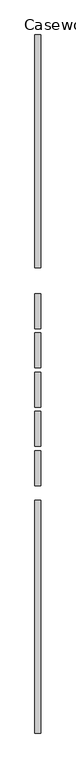
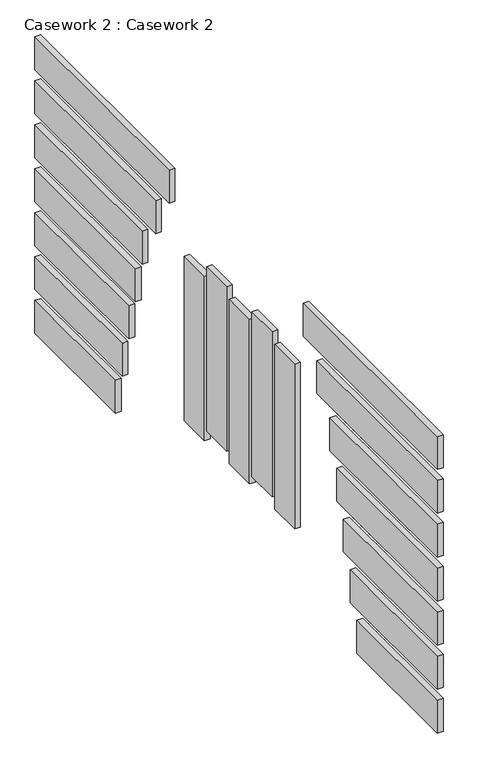
"""IFC4 building model written with IfcOpenShell, lengths in millimetres: furniture geometry, Casework 2 : Casework 2."""

from ifc_helpers import new_model, si_unit, frame, origin, place, context, project, spatial, polyline, outline, extrude, source, transform, mapped, element, save


def casework_2_casework_2_b74305db(model_context):
    return source(origin(), model_context, "Body", "SweptSolid", [
        extrude(outline(polyline([(2710.0501403, -5188.755389), (2710.0501403, -6204.755389), (2684.6501403, -6204.755389), (2684.6501403, -5188.755389), (2710.0501403, -5188.755389)])), frame((0.0, 0.0, 1234.9299166), z_axis=(0.0, 0.0, 1.0), x_axis=(1.0, 0.0, 0.0)), (0.0, 0.0, 1.0), 152.4),
        extrude(outline(polyline([(2710.0501403, -5290.355389), (2710.0501403, -6204.755389), (2684.6501403, -6204.755389), (2684.6501403, -5290.355389), (2710.0501403, -5290.355389)])), frame((0.0, 0.0, 1031.7299166), z_axis=(0.0, 0.0, 1.0), x_axis=(1.0, 0.0, 0.0)), (0.0, 0.0, 1.0), 152.4),
        extrude(outline(polyline([(2710.0501403, -5391.955389), (2710.0501403, -6204.755389), (2684.6501403, -6204.755389), (2684.6501403, -5391.955389), (2710.0501403, -5391.955389)])), frame((0.0, 0.0, 828.5299166), z_axis=(0.0, 0.0, 1.0), x_axis=(1.0, 0.0, 0.0)), (0.0, 0.0, 1.0), 152.4),
        extrude(outline(polyline([(2710.0501403, -5442.755389), (2710.0501403, -6204.755389), (2684.6501403, -6204.755389), (2684.6501403, -5442.755389), (2710.0501403, -5442.755389)])), frame((0.0, 0.0, 625.3299166), z_axis=(0.0, 0.0, 1.0), x_axis=(1.0, 0.0, 0.0)), (0.0, 0.0, 1.0), 152.4),
        extrude(outline(polyline([(2710.0501403, -5493.555389), (2710.0501403, -6204.755389), (2684.6501403, -6204.755389), (2684.6501403, -5493.555389), (2710.0501403, -5493.555389)])), frame((0.0, 0.0, 422.1299166), z_axis=(0.0, 0.0, 1.0), x_axis=(1.0, 0.0, 0.0)), (0.0, 0.0, 1.0), 152.4),
        extrude(outline(polyline([(2710.0501403, -5544.355389), (2710.0501403, -6204.755389), (2684.6501403, -6204.755389), (2684.6501403, -5544.355389), (2710.0501403, -5544.355389)])), frame((0.0, 0.0, 218.9299166), z_axis=(0.0, 0.0, 1.0), x_axis=(1.0, 0.0, 0.0)), (0.0, 0.0, 1.0), 152.4),
        extrude(outline(polyline([(2710.0501403, -5595.155389), (2710.0501403, -6204.755389), (2684.6501403, -6204.755389), (2684.6501403, -5595.155389), (2710.0501403, -5595.155389)])), frame((0.0, 0.0, 15.7299166), z_axis=(0.0, 0.0, 1.0), x_axis=(1.0, 0.0, 0.0)), (0.0, 0.0, 1.0), 152.4),
        extrude(outline(polyline([(2710.0501403, -3156.755389), (2710.0501403, -4172.755389), (2684.6501403, -4172.755389), (2684.6501403, -3156.755389), (2710.0501403, -3156.755389)])), frame((0.0, 0.0, 1234.9299166), z_axis=(0.0, 0.0, 1.0), x_axis=(1.0, 0.0, 0.0)), (0.0, 0.0, 1.0), 152.4),
        extrude(outline(polyline([(2710.0501403, -3156.755389), (2710.0501403, -4071.155389), (2684.6501403, -4071.155389), (2684.6501403, -3156.755389), (2710.0501403, -3156.755389)])), frame((0.0, 0.0, 1031.7299166), z_axis=(0.0, 0.0, 1.0), x_axis=(1.0, 0.0, 0.0)), (0.0, 0.0, 1.0), 152.4),
        extrude(outline(polyline([(2710.0501403, -3156.755389), (2710.0501403, -3969.555389), (2684.6501403, -3969.555389), (2684.6501403, -3156.755389), (2710.0501403, -3156.755389)])), frame((0.0, 0.0, 828.5299166), z_axis=(0.0, 0.0, 1.0), x_axis=(1.0, 0.0, 0.0)), (0.0, 0.0, 1.0), 152.4),
        extrude(outline(polyline([(2710.0501403, -3156.755389), (2710.0501403, -3918.755389), (2684.6501403, -3918.755389), (2684.6501403, -3156.755389), (2710.0501403, -3156.755389)])), frame((0.0, 0.0, 625.3299166), z_axis=(0.0, 0.0, 1.0), x_axis=(1.0, 0.0, 0.0)), (0.0, 0.0, 1.0), 152.4),
        extrude(outline(polyline([(2710.0501403, -3156.755389), (2710.0501403, -3867.955389), (2684.6501403, -3867.955389), (2684.6501403, -3156.755389), (2710.0501403, -3156.755389)])), frame((0.0, 0.0, 422.1299166), z_axis=(0.0, 0.0, 1.0), x_axis=(1.0, 0.0, 0.0)), (0.0, 0.0, 1.0), 152.4),
        extrude(outline(polyline([(2710.0501403, -3156.755389), (2710.0501403, -3817.155389), (2684.6501403, -3817.155389), (2684.6501403, -3156.755389), (2710.0501403, -3156.755389)])), frame((0.0, 0.0, 218.9299166), z_axis=(0.0, 0.0, 1.0), x_axis=(1.0, 0.0, 0.0)), (0.0, 0.0, 1.0), 152.4),
        extrude(outline(polyline([(2710.0501403, -3156.755389), (2710.0501403, -3766.355389), (2684.6501403, -3766.355389), (2684.6501403, -3156.755389), (2710.0501403, -3156.755389)])), frame((0.0, 0.0, 15.7299166), z_axis=(0.0, 0.0, 1.0), x_axis=(1.0, 0.0, 0.0)), (0.0, 0.0, 1.0), 152.4),
        extrude(outline(polyline([(2710.0501403, -4972.4709476), (2710.0501403, -5124.8709476), (2684.6501403, -5124.8709476), (2684.6501403, -4972.4709476), (2710.0501403, -4972.4709476)])), frame((0.0, 0.0, 304.8), z_axis=(0.0, 0.0, 1.0), x_axis=(1.0, 0.0, 0.0)), (0.0, 0.0, 1.0), 762.0),
        extrude(outline(polyline([(2710.0501403, -4800.7293357), (2710.0501403, -4953.1293357), (2684.6501403, -4953.1293357), (2684.6501403, -4800.7293357), (2710.0501403, -4800.7293357)])), frame((0.0, 0.0, 350.8180262), z_axis=(0.0, 0.0, 1.0), x_axis=(1.0, 0.0, 0.0)), (0.0, 0.0, 1.0), 762.0),
        extrude(outline(polyline([(2710.0501403, -4628.9877238), (2710.0501403, -4781.3877238), (2684.6501403, -4781.3877238), (2684.6501403, -4628.9877238), (2710.0501403, -4628.9877238)])), frame((0.0, 0.0, 304.8), z_axis=(0.0, 0.0, 1.0), x_axis=(1.0, 0.0, 0.0)), (0.0, 0.0, 1.0), 762.0),
        extrude(outline(polyline([(2710.0501403, -4457.2461119), (2710.0501403, -4609.6461119), (2684.6501403, -4609.6461119), (2684.6501403, -4457.2461119), (2710.0501403, -4457.2461119)])), frame((0.0, 0.0, 350.8180262), z_axis=(0.0, 0.0, 1.0), x_axis=(1.0, 0.0, 0.0)), (0.0, 0.0, 1.0), 762.0),
        extrude(outline(polyline([(2710.0501403, -4287.7307459), (2710.0501403, -4440.1307459), (2684.6501403, -4440.1307459), (2684.6501403, -4287.7307459), (2710.0501403, -4287.7307459)])), frame((0.0, 0.0, 297.1768043), z_axis=(0.0, 0.0, 1.0), x_axis=(1.0, 0.0, 0.0)), (0.0, 0.0, 1.0), 762.0),
    ])


if __name__ == "__main__":
    model = new_model("IFC4")
    model_context = context("Model", 3, world=origin())
    ifc_project = project(units=[si_unit("LENGTHUNIT", "METRE", prefix="MILLI")], contexts=[model_context])
    site = spatial("IfcSite", under=ifc_project)
    building = spatial("IfcBuilding", under=site)
    placement = place(None, origin())
    casework_2_casework_2_shape = casework_2_casework_2_b74305db(model_context)
    element("IfcFurniture", 1, ObjectType="Casework 2 : Casework 2", at=placement, inside=building, context=model_context, shape_type="MappedRepresentation", body=[
        mapped(casework_2_casework_2_shape, transform((0.0, 0.0, 0.0), x_axis=(1.0, 0.0, 0.0), y_axis=(0.0, 1.0, 0.0), z_axis=(0.0, 0.0, 1.0))),
    ])
    save(model, "model.ifc")

# Revit data of these elements
# Element 1 (IfcFurniture, "Casework 2 : Casework 2")
#   Materials on its faces: "Clad - White"
# Materials
#   "Clad - White": class "Wood", colour RGB 242 242 238, transparency 0, Cost = 0
